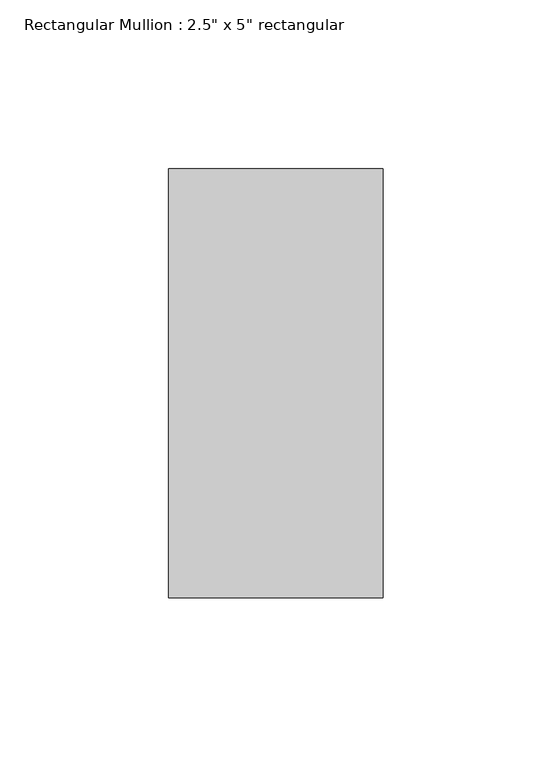
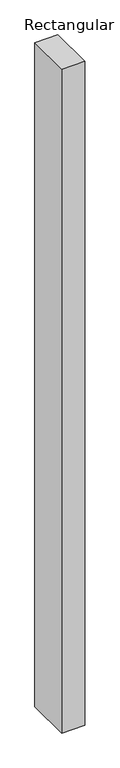
"""IFC4 building model written with IfcOpenShell, lengths in millimetres: member geometry."""

from ifc_helpers import new_model, si_unit, frame, origin, place, context, project, spatial, polyline, outline, extrude, source, transform, mapped, element, save


def member_c304ec9f(model_context):
    return source(origin(), model_context, "Body", "SweptSolid", [
        extrude(outline(polyline([(0.0, 63.5), (0.0, -63.5), (-63.5, -63.5), (-63.5, 63.5), (0.0, 63.5)])), frame((0.0, 0.0, -1931.193737), z_axis=(0.0, 0.0, 1.0), x_axis=(1.0, 0.0, 0.0)), (0.0, 0.0, 1.0), 1931.193737),
    ])


if __name__ == "__main__":
    model = new_model("IFC4")
    model_context = context("Model", 3, world=origin())
    ifc_project = project(units=[si_unit("LENGTHUNIT", "METRE", prefix="MILLI")], contexts=[model_context])
    site = spatial("IfcSite", under=ifc_project)
    building = spatial("IfcBuilding", under=site)
    placement = place(None, origin())
    member_shape = member_c304ec9f(model_context)
    element("IfcMember", 1, ObjectType="Rectangular Mullion : 2.5\" x 5\" rectangular", at=placement, inside=building, context=model_context, shape_type="MappedRepresentation", body=[
        mapped(member_shape, transform((0.0, 0.0, 0.0), x_axis=(1.0, 0.0, 0.0), y_axis=(0.0, 1.0, 0.0), z_axis=(0.0, 0.0, 1.0))),
    ])
    save(model, "model.ifc")

# Revit data of these elements
# Type "Rectangular Mullion : 2.5\" x 5\" rectangular"
#   built-in parameter 1007304 = 0.416667 (stored number, unit not read)
#   built-in parameter 1007301 = 0.104167 (stored number, unit not read)
#   built-in parameter 1007300 = 0.104167 (stored number, unit not read)
# Element 1 (IfcMember, "Rectangular Mullion : 2.5\" x 5\" rectangular")
#   Materials on its faces: "Aluminum"
# Materials
#   "Aluminum": class "Metal", colour RGB 247 247 247, transparency 0, Description = "Aluminum 6061", Cost = 0
